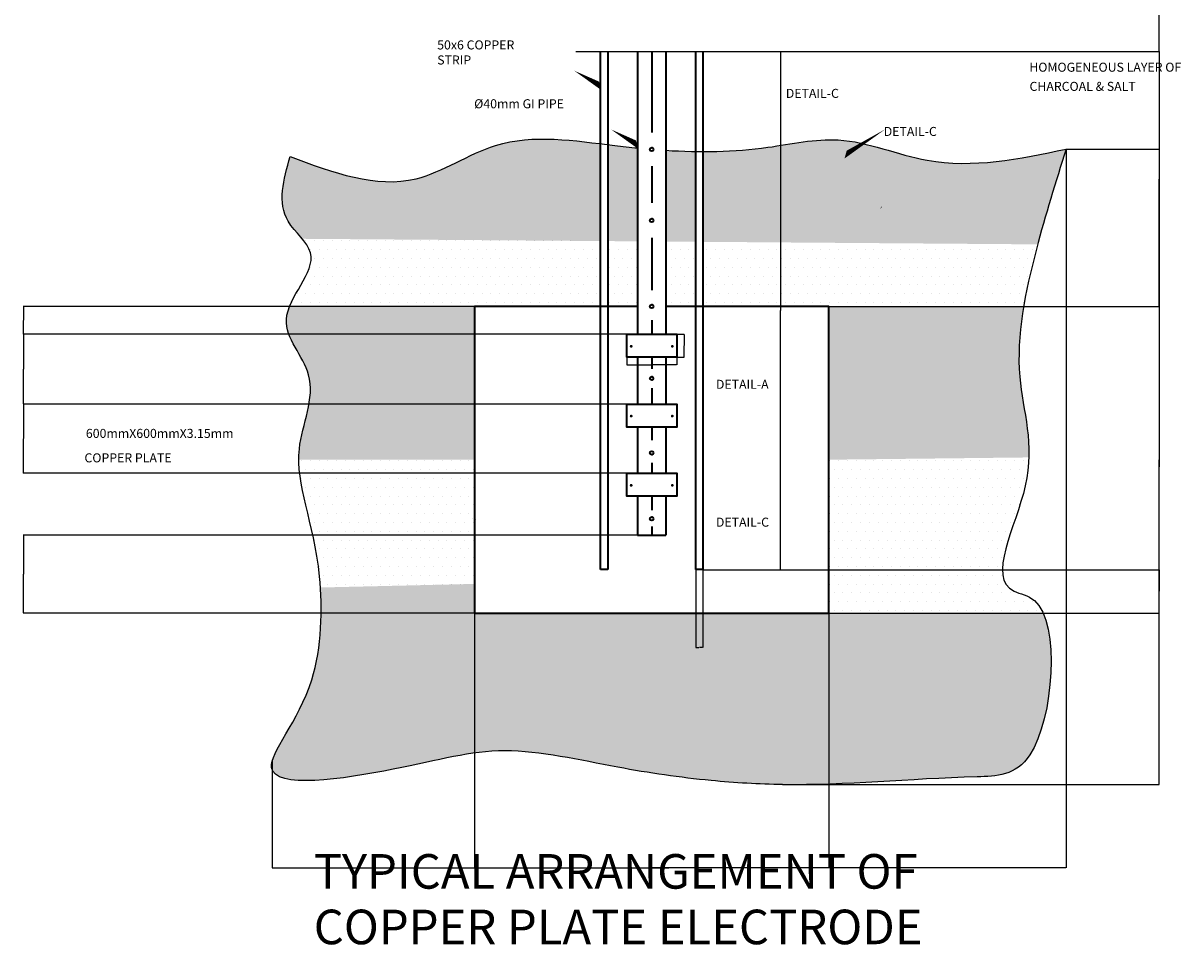
# Model space of a CAD drawing. Units: inches. Extents: x -514 to 1130, y -1450 to 978.
# Tile 1 of 2: x -514 to 1130, y -1450 to -141. Entities that reach past the tile are written whole.
import ezdxf

# ---------------------------------------------------------------- set-up
doc = ezdxf.new("R2010")
doc.units = ezdxf.units.IN
doc.header["$MEASUREMENT"] = 0
for name, color, linetype, lineweight in [('A-ANNO-DIMS', 2, 'Continuous', 18), ('C-TOPO', 3, 'Continuous', 25), ('C-TOPO-PATT', 252, 'Continuous', 13), ('E-ANNO-LEAD', 2, 'Continuous', 18), ('E-ANNO-TEXT', 7, 'Continuous', 18), ('E-GRND', 1, 'Continuous', 35)]:
    doc.layers.add(name, color=color, linetype=linetype, lineweight=lineweight)
doc.styles.get("Standard").update_dxf_attribs({"font": 'arial.ttf'})
doc.dimstyles.get("Standard").update_dxf_attribs({"dimtxt": 0.18, "dimasz": 0.18, "dimexe": 0.18, "dimexo": 0.0625, "dimgap": 0.09, "dimtad": 0, "dimtih": 1, "dimtoh": 1, "dimdec": 4, "dimzin": 0, "dimdsep": 46, "dimtxsty": 'Standard', "dimcen": 0.09, "dimadec": 0, "dimazin": 0, "dimtfac": 1, "dimtdec": 4, "dimtofl": 0, "dimtmove": 0, "dimatfit": 3, "dimfxl": 1, "dimtolj": 1, "dimtzin": 0, "dimarcsym": 0})

# ---------------------------------------------------------------- blocks, each defined once
blk = doc.blocks.new('CLAMP-PIPE')
blk.add_lwpolyline([(342.9, -582.6), (413.9, -582.6), (413.9, -615.2), (342.9, -615.2)], close=True)
at = {"const_width": 1.95}
for points in [[(348.3, -599.7, 1), (350.3, -599.7, 1)], [(406.7, -599.7, 1), (408.6, -599.7, 1)]]:
    blk.add_lwpolyline(points, format="xyb", close=True, dxfattribs=at)
blk = doc.blocks.new('COPPER-STRIP-50X6')
blk.add_line((10, 0), (0, 0))
for points in [[(0, 0), (0, 736)], [(10, 736), (10, 0)]]:
    blk.add_lwpolyline(points)
blk = doc.blocks.new('*D3')
at = {"layer": 'A-ANNO-DIMS', "color": 0, "lineweight": -2, "transparency": 16777216}
for p, q in [((342.9, -615.3), (342.9, -626)), ((413.9, -615.3), (413.9, -626)), ((343.1, -625.8), (377.1, -625.8)), ((413.7, -625.8), (379.7, -625.8))]:
    blk.add_line(p, q, dxfattribs=at)
at = {"layer": 'A-ANNO-DIMS', "color": 0, "transparency": 16777216}
for points in [[(343.1, -625.8), (343.1, -625.9), (342.9, -625.8)], [(413.7, -625.8), (413.7, -625.9), (413.9, -625.8)]]:
    blk.add_solid(points, dxfattribs=at)
at = {"layer": 'Defpoints', "color": 0, "transparency": 16777216}
for p in [(342.9, -615.2), (413.9, -615.2), (413.9, -625.8)]:
    blk.add_point(p, dxfattribs=at)
at = {"layer": 'A-ANNO-DIMS', "color": 0, "transparency": 16777216, "insert": (378.4, -625.8), "char_height": 0.18, "attachment_point": 5}
blk.add_mtext('\\A1;PIPE CLAMP 71 TYP.', dxfattribs=at)
blk = doc.blocks.new('*D4')
at = {"layer": 'A-ANNO-DIMS', "color": 0, "lineweight": -2, "transparency": 16777216}
for p, q in [((413.9, -582.6), (424.7, -582.6)), ((424.5, -582.8), (424.5, -598.7)), ((424.5, -615), (424.5, -599.1)), ((413.9, -615.2), (424.7, -615.2))]:
    blk.add_line(p, q, dxfattribs=at)
at = {"layer": 'A-ANNO-DIMS', "color": 0, "transparency": 16777216}
for points in [[(424.5, -582.8), (424.5, -582.8), (424.5, -582.6)], [(424.5, -615), (424.5, -615), (424.5, -615.2)]]:
    blk.add_solid(points, dxfattribs=at)
at = {"layer": 'Defpoints', "color": 0, "transparency": 16777216}
for p in [(413.9, -582.6), (424.5, -582.6), (413.9, -615.2)]:
    blk.add_point(p, dxfattribs=at)
at = {"layer": 'A-ANNO-DIMS', "color": 0, "transparency": 16777216, "insert": (424.5, -598.9), "char_height": 0.18, "attachment_point": 5}
blk.add_mtext('\\A1;33 TYP.', dxfattribs=at)
blk = doc.blocks.new('*D5')
at = {"layer": 'A-ANNO-DIMS', "color": 0, "lineweight": -2, "transparency": 16777216}
for p, q in [((451, -180.9), (561.5, -180.9)), ((561.3, -181.1), (561.3, -548.7)), ((561.3, -916.7), (561.3, -549.1)), ((451, -916.9), (561.5, -916.9))]:
    blk.add_line(p, q, dxfattribs=at)
at = {"layer": 'A-ANNO-DIMS', "color": 0, "transparency": 16777216}
for points in [[(561.3, -181.1), (561.3, -181.1), (561.3, -180.9)], [(561.3, -916.7), (561.3, -916.7), (561.3, -916.9)]]:
    blk.add_solid(points, dxfattribs=at)
at = {"layer": 'Defpoints', "color": 0, "transparency": 16777216}
for p in [(450.9, -180.9), (561.3, -180.9), (450.9, -916.9)]:
    blk.add_point(p, dxfattribs=at)
at = {"layer": 'A-ANNO-DIMS', "color": 0, "transparency": 16777216, "insert": (561.3, -548.9), "char_height": 0.18, "attachment_point": 5}
blk.add_mtext('\\A1;50X6 COPPER STRIP 736 TYP.', dxfattribs=at)
blk = doc.blocks.new('*D6')
at = {"layer": 'A-ANNO-DIMS', "color": 0, "lineweight": -2, "transparency": 16777216}
for p, q in [((440.9, -917), (440.9, -1027.5)), ((450.9, -917), (450.9, -1027.5)), ((441.1, -1027.3), (445.4, -1027.3)), ((450.7, -1027.3), (446.4, -1027.3))]:
    blk.add_line(p, q, dxfattribs=at)
at = {"layer": 'A-ANNO-DIMS', "color": 0, "transparency": 16777216}
for points in [[(441.1, -1027.3), (441.1, -1027.3), (440.9, -1027.3)], [(450.7, -1027.3), (450.7, -1027.3), (450.9, -1027.3)]]:
    blk.add_solid(points, dxfattribs=at)
at = {"layer": 'Defpoints', "color": 0, "transparency": 16777216}
for p in [(440.9, -916.9), (450.9, -916.9), (450.9, -1027.3)]:
    blk.add_point(p, dxfattribs=at)
at = {"layer": 'A-ANNO-DIMS', "color": 0, "transparency": 16777216, "insert": (445.9, -1027.3), "char_height": 0.18, "attachment_point": 5}
blk.add_mtext('\\A1;10 TYP.', dxfattribs=at)
blk = doc.blocks.new('*D22')
at = {"layer": 'A-ANNO-DIMS', "color": 0, "lineweight": -2, "transparency": 16777216}
for p, q in [((491.3, 109.1), (1099, 109.1)), ((1098.9, 108.9), (1098.9, -35.7)), ((1098.9, -180.7), (1098.9, -36.1)), ((491.3, -180.9), (1099, -180.9))]:
    blk.add_line(p, q, dxfattribs=at)
at = {"layer": 'A-ANNO-DIMS', "color": 0, "transparency": 16777216}
for points in [[(1098.8, 108.9), (1098.9, 108.9), (1098.9, 109.1)], [(1098.8, -180.7), (1098.9, -180.7), (1098.9, -180.9)]]:
    blk.add_solid(points, dxfattribs=at)
at = {"layer": 'Defpoints', "color": 0, "transparency": 16777216}
for p in [(491.2, 109.1), (491.2, -180.9), (1098.9, -180.9)]:
    blk.add_point(p, dxfattribs=at)
at = {"layer": 'A-ANNO-DIMS', "color": 0, "transparency": 16777216, "insert": (1098.9, -35.9), "char_height": 0.18, "attachment_point": 5}
blk.add_mtext('\\A1;290', dxfattribs=at)
blk = doc.blocks.new('*D26')
at = {"layer": 'A-ANNO-DIMS', "color": 0, "lineweight": -2, "transparency": 16777216}
for p, q in [((126.9, -978.5), (126.9, -1340.3)), ((629.9, -978.5), (629.9, -1340.3)), ((127.1, -1340.1), (378.1, -1340.1)), ((629.7, -1340.1), (378.7, -1340.1))]:
    blk.add_line(p, q, dxfattribs=at)
at = {"layer": 'A-ANNO-DIMS', "color": 0, "transparency": 16777216}
for points in [[(127.1, -1340), (127.1, -1340.1), (126.9, -1340.1)], [(629.7, -1340), (629.7, -1340.1), (629.9, -1340.1)]]:
    blk.add_solid(points, dxfattribs=at)
at = {"layer": 'Defpoints', "color": 0, "transparency": 16777216}
for p in [(126.9, -978.5), (629.9, -978.5), (629.9, -1340.1)]:
    blk.add_point(p, dxfattribs=at)
at = {"layer": 'A-ANNO-DIMS', "color": 0, "transparency": 16777216, "insert": (378.4, -1340.1), "char_height": 0.18, "attachment_point": 5}
blk.add_mtext('\\A1;503', dxfattribs=at)
blk = doc.blocks.new('*D27')
at = {"layer": 'A-ANNO-DIMS', "color": 0, "lineweight": -2, "transparency": 16777216}
for p, q in [((630, -543), (1099, -543)), ((1098.9, -543.2), (1098.9, -760.6)), ((1098.9, -978.3), (1098.9, -760.9)), ((630, -978.5), (1099, -978.5))]:
    blk.add_line(p, q, dxfattribs=at)
at = {"layer": 'A-ANNO-DIMS', "color": 0, "transparency": 16777216}
for points in [[(1098.8, -543.2), (1098.9, -543.2), (1098.9, -543)], [(1098.8, -978.3), (1098.9, -978.3), (1098.9, -978.5)]]:
    blk.add_solid(points, dxfattribs=at)
at = {"layer": 'Defpoints', "color": 0, "transparency": 16777216}
for p in [(629.9, -543), (629.9, -978.5), (1098.9, -978.5)]:
    blk.add_point(p, dxfattribs=at)
at = {"layer": 'A-ANNO-DIMS', "color": 0, "transparency": 16777216, "insert": (1098.9, -760.8), "char_height": 0.18, "attachment_point": 5}
blk.add_mtext('\\A1;435.4', dxfattribs=at)
blk = doc.blocks.new('*D28')
at = {"layer": 'A-ANNO-DIMS', "color": 0, "lineweight": -2, "transparency": 16777216}
for p, q in [((491.3, -180.9), (1099, -180.9)), ((1098.9, -181.1), (1098.9, -361.8)), ((1098.9, -542.9), (1098.9, -362.2)), ((630, -543), (1099, -543))]:
    blk.add_line(p, q, dxfattribs=at)
at = {"layer": 'A-ANNO-DIMS', "color": 0, "transparency": 16777216}
for points in [[(1098.8, -181.1), (1098.9, -181.1), (1098.9, -180.9)], [(1098.8, -542.9), (1098.9, -542.9), (1098.9, -543)]]:
    blk.add_solid(points, dxfattribs=at)
at = {"layer": 'Defpoints', "color": 0, "transparency": 16777216}
for p in [(491.2, -180.9), (629.9, -543), (1098.9, -543)]:
    blk.add_point(p, dxfattribs=at)
at = {"layer": 'A-ANNO-DIMS', "color": 0, "transparency": 16777216, "insert": (1098.9, -362), "char_height": 0.18, "attachment_point": 5}
blk.add_mtext('\\A1;362.14', dxfattribs=at)
blk = doc.blocks.new('*D29')
at = {"layer": 'A-ANNO-DIMS', "color": 0, "lineweight": -2, "transparency": 16777216}
for p, q in [((451, -916.9), (1099, -916.9)), ((1098.9, -917.1), (1098.9, -947.5)), ((1098.9, -978.3), (1098.9, -947.9)), ((630, -978.5), (1099, -978.5))]:
    blk.add_line(p, q, dxfattribs=at)
at = {"layer": 'A-ANNO-DIMS', "color": 0, "transparency": 16777216}
for points in [[(1098.8, -917.1), (1098.9, -917.1), (1098.9, -916.9)], [(1098.8, -978.3), (1098.9, -978.3), (1098.9, -978.5)]]:
    blk.add_solid(points, dxfattribs=at)
at = {"layer": 'Defpoints', "color": 0, "transparency": 16777216}
for p in [(450.9, -916.9), (629.9, -978.5), (1098.9, -978.5)]:
    blk.add_point(p, dxfattribs=at)
at = {"layer": 'A-ANNO-DIMS', "color": 0, "transparency": 16777216, "insert": (1098.9, -947.7), "char_height": 0.18, "attachment_point": 5}
blk.add_mtext('\\A1;61.58', dxfattribs=at)
blk = doc.blocks.new('*D30')
at = {"layer": 'A-ANNO-DIMS', "color": 0, "lineweight": -2, "transparency": 16777216}
for p, q in [((126.9, -543), (-513.8, -543)), ((-513.7, -543.2), (-513.7, -562.7)), ((-513.7, -582.5), (-513.7, -563)), ((342.9, -582.6), (-513.8, -582.6))]:
    blk.add_line(p, q, dxfattribs=at)
at = {"layer": 'A-ANNO-DIMS', "color": 0, "transparency": 16777216}
for points in [[(-513.7, -543.2), (-513.6, -543.2), (-513.7, -543)], [(-513.7, -582.5), (-513.6, -582.5), (-513.7, -582.6)]]:
    blk.add_solid(points, dxfattribs=at)
at = {"layer": 'Defpoints', "color": 0, "transparency": 16777216}
for p in [(126.9, -543), (-513.7, -582.6), (342.9, -582.6)]:
    blk.add_point(p, dxfattribs=at)
at = {"layer": 'A-ANNO-DIMS', "color": 0, "transparency": 16777216, "insert": (-513.7, -562.8), "char_height": 0.18, "attachment_point": 5}
blk.add_mtext('\\A1;39.594', dxfattribs=at)
blk = doc.blocks.new('*D31')
at = {"layer": 'A-ANNO-DIMS', "color": 0, "lineweight": -2, "transparency": 16777216}
for p, q in [((342.9, -582.6), (-513.8, -582.6)), ((-513.7, -582.8), (-513.7, -632)), ((-513.7, -681.6), (-513.7, -632.4)), ((342.9, -681.8), (-513.8, -681.8))]:
    blk.add_line(p, q, dxfattribs=at)
at = {"layer": 'A-ANNO-DIMS', "color": 0, "transparency": 16777216}
for points in [[(-513.7, -582.8), (-513.6, -582.8), (-513.7, -582.6)], [(-513.7, -681.6), (-513.6, -681.6), (-513.7, -681.8)]]:
    blk.add_solid(points, dxfattribs=at)
at = {"layer": 'Defpoints', "color": 0, "transparency": 16777216}
for p in [(342.9, -582.6), (-513.7, -681.8), (342.9, -681.8)]:
    blk.add_point(p, dxfattribs=at)
at = {"layer": 'A-ANNO-DIMS', "color": 0, "transparency": 16777216, "insert": (-513.7, -632.2), "char_height": 0.18, "attachment_point": 5}
blk.add_mtext('\\A1;99.12', dxfattribs=at)
blk = doc.blocks.new('*D32')
at = {"layer": 'A-ANNO-DIMS', "color": 0, "lineweight": -2, "transparency": 16777216}
for p, q in [((342.9, -681.8), (-513.8, -681.8)), ((-513.7, -681.9), (-513.7, -730.8)), ((-513.7, -779.9), (-513.7, -731.1)), ((342.9, -780.1), (-513.8, -780.1))]:
    blk.add_line(p, q, dxfattribs=at)
at = {"layer": 'A-ANNO-DIMS', "color": 0, "transparency": 16777216}
for points in [[(-513.7, -681.9), (-513.6, -681.9), (-513.7, -681.8)], [(-513.7, -779.9), (-513.6, -779.9), (-513.7, -780.1)]]:
    blk.add_solid(points, dxfattribs=at)
at = {"layer": 'Defpoints', "color": 0, "transparency": 16777216}
for p in [(342.9, -681.8), (-513.7, -780.1), (342.9, -780.1)]:
    blk.add_point(p, dxfattribs=at)
at = {"layer": 'A-ANNO-DIMS', "color": 0, "transparency": 16777216, "insert": (-513.7, -730.9), "char_height": 0.18, "attachment_point": 5}
blk.add_mtext('\\A1;98.37', dxfattribs=at)
blk = doc.blocks.new('*D33')
at = {"layer": 'A-ANNO-DIMS', "color": 0, "lineweight": -2, "transparency": 16777216}
for p, q in [((358.3, -868.1), (-513.8, -868.1)), ((-513.7, -868.3), (-513.7, -923.1)), ((-513.7, -978.3), (-513.7, -923.5)), ((126.9, -978.5), (-513.8, -978.5))]:
    blk.add_line(p, q, dxfattribs=at)
at = {"layer": 'A-ANNO-DIMS', "color": 0, "transparency": 16777216}
for points in [[(-513.7, -868.3), (-513.6, -868.3), (-513.7, -868.1)], [(-513.7, -978.3), (-513.6, -978.3), (-513.7, -978.5)]]:
    blk.add_solid(points, dxfattribs=at)
at = {"layer": 'Defpoints', "color": 0, "transparency": 16777216}
for p in [(358.4, -868.1), (-513.7, -978.5), (126.9, -978.5)]:
    blk.add_point(p, dxfattribs=at)
at = {"layer": 'A-ANNO-DIMS', "color": 0, "transparency": 16777216, "insert": (-513.7, -923.3), "char_height": 0.18, "attachment_point": 5}
blk.add_mtext('\\A1;110.35', dxfattribs=at)
blk = doc.blocks.new('*D34')
at = {"layer": 'A-ANNO-DIMS', "color": 0, "lineweight": -2, "transparency": 16777216}
for p, q in [((966.7, -319.9), (966.7, -1340.3)), ((-160.5, -1188.9), (-160.5, -1340.3)), ((-160.4, -1340.1), (402.6, -1340.1)), ((966.5, -1340.1), (403.6, -1340.1))]:
    blk.add_line(p, q, dxfattribs=at)
at = {"layer": 'A-ANNO-DIMS', "color": 0, "transparency": 16777216}
for points in [[(-160.4, -1340), (-160.4, -1340.1), (-160.5, -1340.1)], [(966.5, -1340), (966.5, -1340.1), (966.7, -1340.1)]]:
    blk.add_solid(points, dxfattribs=at)
at = {"layer": 'Defpoints', "color": 0, "transparency": 16777216}
for p in [(966.7, -319.8), (-160.5, -1188.9), (966.7, -1340.1)]:
    blk.add_point(p, dxfattribs=at)
at = {"layer": 'A-ANNO-DIMS', "color": 0, "transparency": 16777216, "insert": (403.1, -1340.1), "char_height": 0.18, "attachment_point": 5}
blk.add_mtext('\\A1;1127.3', dxfattribs=at)
blk = doc.blocks.new('*D35')
at = {"layer": 'A-ANNO-DIMS', "color": 0, "lineweight": -2, "transparency": 16777216}
for p, q in [((966.8, -319.8), (1099, -319.8)), ((1098.9, -320), (1098.9, -770.8)), ((1098.9, -1221.9), (1098.9, -771.1)), ((564.3, -1222.1), (1099, -1222.1))]:
    blk.add_line(p, q, dxfattribs=at)
at = {"layer": 'A-ANNO-DIMS', "color": 0, "transparency": 16777216}
for points in [[(1098.8, -320), (1098.9, -320), (1098.9, -319.8)], [(1098.8, -1221.9), (1098.9, -1221.9), (1098.9, -1222.1)]]:
    blk.add_solid(points, dxfattribs=at)
at = {"layer": 'Defpoints', "color": 0, "transparency": 16777216}
for p in [(966.7, -319.8), (564.2, -1222.1), (1098.9, -1222.1)]:
    blk.add_point(p, dxfattribs=at)
at = {"layer": 'A-ANNO-DIMS', "color": 0, "transparency": 16777216, "insert": (1098.9, -770.9), "char_height": 0.18, "attachment_point": 5}
blk.add_mtext('\\A1;902.3', dxfattribs=at)

msp = doc.modelspace()

# ---------------------------------------------------------------- hatches: boundary and pattern name
at = {"layer": 'C-TOPO-PATT'}
h = msp.add_hatch(dxfattribs=at)
h.set_pattern_fill('HEX', color=256, scale=60)
edge = h.paths.add_edge_path()
edge.add_spline(control_points=[(305.9114, -312.0843), (255.1866, -305.7764), (162.1476, -294.9931), (28.4437, -390.9059), (-73.917, -352.9564), (-135.0278, -330.3001), (-144.1924, -363.0231), (-156.3777, -406.5315), (-124.607, -439.0103), (-117.9173, -447.0708)], knot_values=[2558.576308896, 2558.576308896, 2558.576308896, 2558.576308896, 2707.976967101, 2830.531301613, 3012.092961341, 3012.092961341, 3012.092961341, 3104.06054613, 3134.372709078, 3134.372709078, 3134.372709078, 3134.372709078], degree=3, periodic=0)
edge.add_line((-117.9173, -447.0708), (305.9114, -450.2757))
edge.add_line((305.9114, -450.2757), (305.9114, -312.0843))
edge = h.paths.add_edge_path()
edge.add_spline(control_points=[(926.4196, -454.9679), (938.7739, -408.7375), (952.75, -364.2656), (966.726, -319.7938)], knot_values=[0, 0, 0, 0, 141.175598989, 141.175598989, 141.175598989, 141.175598989], degree=3, periodic=0)
edge.add_spline(control_points=[(966.726, -319.7938), (900.3974, -333.5642), (790.659, -356.3469), (653.584, -294.712), (545.7543, -319.617), (481.7435, -323.2948), (450.9114, -323.2008)], knot_values=[3278.625747001, 3278.625747001, 3278.625747001, 3278.625747001, 3476.465744458, 3605.945645556, 3706.416880749, 3799.313199321, 3799.313199321, 3799.313199321, 3799.313199321], degree=3, periodic=0)
edge.add_line((450.9114, -323.2008), (450.9114, -451.3722))
edge.add_line((450.9114, -451.3722), (926.4196, -454.9679))
edge = h.paths.add_edge_path()
edge.add_spline(control_points=[(358.4114, -318.1134), (347.593, -317.0483), (333.4463, -315.4827), (319.2248, -313.738), (315.9114, -313.3278)], knot_values=[3144.196564241, 3144.196564241, 3144.196564241, 3144.196564241, 3176.40431904, 3186.1768941, 3186.1768941, 3186.1768941, 3186.1768941], degree=3, periodic=0)
edge.add_line((315.9114, -313.3278), (315.9114, -450.3514))
edge.add_line((315.9114, -450.3514), (358.4114, -450.6727))
edge.add_line((358.4114, -450.6727), (358.4114, -318.1134))
edge = h.paths.add_edge_path()
edge.add_spline(control_points=[(440.9114, -323.106), (426.7733, -322.8825), (412.6134, -322.2848), (398.4114, -321.3836)], knot_values=[3226.015463929, 3226.015463929, 3226.015463929, 3226.015463929, 3268.585625788, 3268.585625788, 3268.585625788, 3268.585625788], degree=3, periodic=0)
edge.add_line((398.4114, -321.3836), (398.4114, -450.9752))
edge.add_line((398.4114, -450.9752), (440.9114, -451.2966))
edge.add_line((440.9114, -451.2966), (440.9114, -323.106))
edge = h.paths.add_edge_path()
edge.add_spline(control_points=[(913.9671, -757.5216), (915.1505, -715.9834), (894.9887, -650.219), (900.9088, -576.9646), (906.5871, -543.0396)], knot_values=[229.379387274, 229.379387274, 229.379387274, 229.379387274, 348.036394784, 449.372068737, 449.372068737, 449.372068737, 449.372068737], degree=3, periodic=0)
edge.add_line((906.5871, -543.0396), (629.9001, -543.0396))
edge.add_line((629.9001, -543.0396), (629.9001, -760.755))
edge.add_line((629.9001, -760.755), (913.9671, -757.5216))
edge = h.paths.add_edge_path()
edge.add_line((126.9226, -543.0396), (-135.6988, -543.0396))
edge.add_spline(control_points=[(-135.6988, -543.0396), (-138.2127, -549.2256), (-147.596, -582.6879), (-84.3642, -644.6462), (-120.7631, -715.3201), (-122.6941, -755.6416), (-122.6721, -760.8136)], knot_values=[2227.362231503, 2227.362231503, 2227.362231503, 2227.362231503, 2246.486456495, 2331.366553539, 2437.248834262, 2452.791404045, 2452.791404045, 2452.791404045, 2452.791404045], degree=3, periodic=0)
edge.add_line((-122.6721, -760.8136), (126.9226, -760.755))
edge.add_line((126.9226, -760.755), (126.9226, -543.0396))
h = msp.add_hatch(dxfattribs=at)
h.set_pattern_fill('DOTS', color=256, scale=200)
edge = h.paths.add_edge_path()
edge.add_line((305.9114, -450.2757), (-117.9173, -447.0708))
edge.add_spline(control_points=[(-117.9173, -447.0708), (-112.5404, -453.5495), (-92.5209, -481.7059), (-124.9959, -516.7024), (-135.6988, -543.0396)], knot_values=[2452.791404045, 2452.791404045, 2452.791404045, 2452.791404045, 2477.154815033, 2558.576308896, 2558.576308896, 2558.576308896, 2558.576308896], degree=3, periodic=0)
edge.add_line((-135.6988, -543.0396), (126.9226, -543.0396))
edge.add_line((126.9226, -543.0396), (305.9114, -543.0396))
edge.add_line((305.9114, -543.0396), (305.9114, -450.2757))
h = msp.add_hatch(dxfattribs=at)
h.set_pattern_fill('DOTS', color=256, scale=200)
edge = h.paths.add_edge_path()
edge.add_line((126.9226, -760.755), (-122.6721, -760.8136))
edge.add_spline(control_points=[(-122.6721, -760.8136), (-122.4736, -807.4113), (-98.8319, -858.3093), (-92.2406, -936.8365), (-91.8839, -942.218)], knot_values=[2077.226003647, 2077.226003647, 2077.226003647, 2077.226003647, 2217.258049419, 2227.362231503, 2227.362231503, 2227.362231503, 2227.362231503], degree=3, periodic=0)
edge.add_line((-91.8839, -942.218), (126.9226, -937.1171))
edge.add_line((126.9226, -937.1171), (126.9226, -760.755))
edge = h.paths.add_edge_path()
edge.add_spline(control_points=[(934.1175, -978.4705), (930.7904, -971.0144), (919.2875, -954.0087), (844.5148, -943.3117), (905.8885, -838.7284), (913.603, -770.3031), (913.9671, -757.5216)], knot_values=[449.372068737, 449.372068737, 449.372068737, 449.372068737, 466.426239302, 497.199581115, 647.743126183, 684.254466767, 684.254466767, 684.254466767, 684.254466767], degree=3, periodic=0)
edge.add_line((913.9671, -757.5216), (629.9001, -760.755))
edge.add_line((629.9001, -760.755), (629.9001, -978.4705))
edge.add_line((629.9001, -978.4705), (934.1175, -978.4705))
edge = h.paths.add_edge_path()
edge.add_spline(control_points=[(906.5871, -543.0396), (911.1503, -515.7764), (918.1572, -486.1206), (925.8274, -457.184), (926.4196, -454.9679)], knot_values=[141.175598989, 141.175598989, 141.175598989, 141.175598989, 222.611902009, 229.379387274, 229.379387274, 229.379387274, 229.379387274], degree=3, periodic=0)
edge.add_line((926.4196, -454.9679), (450.9114, -451.3722))
edge.add_line((450.9114, -451.3722), (450.9114, -543.0396))
edge.add_line((450.9114, -543.0396), (629.9001, -543.0396))
edge.add_line((629.9001, -543.0396), (906.5871, -543.0396))
h.paths.add_polyline_path([(440.9114, -451.2966), (398.4114, -450.9752), (398.4114, -543.0396), (440.9114, -543.0396)])
h.paths.add_polyline_path([(358.4114, -450.6727), (315.9114, -450.3514), (315.9114, -543.0396), (358.4114, -543.0396)])
h = msp.add_hatch(dxfattribs=at)
h.set_pattern_fill('HEX', color=256, scale=60)
edge = h.paths.add_edge_path()
edge.add_spline(control_points=[(-91.8839, -942.218), (-89.0821, -984.4826), (-95.4593, -1104.845), (-224.3178, -1239.0629), (31.1239, -1200.9077), (163.9896, -1161.2999), (322.5805, -1198.0653), (451.365, -1216.9213), (623.7933, -1227.0137), (765.4968, -1211.2096), (936.7185, -1209.5718), (955.9045, -1027.2952), (934.1175, -978.4705)], knot_values=[684.254466767, 684.254466767, 684.254466767, 684.254466767, 763.608423146, 882.298593781, 1055.253603965, 1215.7522685, 1377.799282437, 1511.646302567, 1613.237961486, 1889.664797207, 1965.551324857, 2077.226003647, 2077.226003647, 2077.226003647, 2077.226003647], degree=3, periodic=0)
edge.add_line((934.1175, -978.4705), (629.9001, -978.4705))
edge.add_line((629.9001, -978.4705), (126.9226, -978.4705))
edge.add_line((126.9226, -978.4705), (126.9226, -937.1171))
edge.add_line((126.9226, -937.1171), (-91.8839, -942.218))

# ---------------------------------------------------------------- linework, layer by layer
at = {"layer": 'C-TOPO'}
msp.add_line((270.9153, -180.8997), (491.2068, -180.8997), dxfattribs=at)
for points, knots in [([(966.726, -319.7938), (952.08, -366.3975), (919.34, -470.5764), (884.9403, -638.4925), (939.3204, -781.759), (844.5148, -943.3117), (961.3814, -960.0307), (943.0119, -1209.5116), (765.4968, -1211.2096), (623.7933, -1227.0137), (451.365, -1216.9213), (322.5805, -1198.0653), (163.9896, -1161.2999), (31.1239, -1200.9077), (-224.3178, -1239.0629), (-91.9498, -1101.1896), (-86.0856, -875.5702), (-145.4693, -763.2908), (-84.3642, -644.6462), (-172.1255, -558.6523), (-76.8768, -476.4137), (-158.8055, -415.2003), (-144.1924, -363.0231), (-135.0278, -330.3001), (-73.917, -352.9564), (28.4437, -390.9059), (167.9249, -290.8487), (279.7902, -309.5449), (347.593, -317.0483), (358.4114, -318.1134)], [0, 0, 0, 0, 147.943084254, 330.715061227, 485.88340932, 636.426954389, 667.200296202, 795.929145557, 871.815673207, 1148.242508928, 1249.834167847, 1383.681187977, 1545.728201914, 1706.226866449, 1879.181876633, 1997.872047268, 2087.330185731, 2242.904801285, 2348.787082008, 2433.667179053, 2534.212897908, 2588.888471844, 2680.856056633, 2680.856056633, 2680.856056633, 2862.417716362, 2984.972050874, 3153.969139301, 3186.1768941, 3186.1768941, 3186.1768941, 3186.1768941]), ([(398.4114, -321.3836), (446.9546, -324.4642), (528.1827, -323.6755), (653.584, -294.712), (790.659, -356.3469), (900.3974, -333.5642), (966.726, -319.7938)], [3226.015463929, 3226.015463929, 3226.015463929, 3226.015463929, 3371.522065573, 3471.993300766, 3601.473201864, 3799.313199321, 3799.313199321, 3799.313199321, 3799.313199321])]:
    msp.add_open_spline(points, degree=3, knots=knots, dxfattribs=at)
at = {"layer": 'E-ANNO-LEAD'}
for points in [[(306.9307, -236.0174, 0, 13.2101, 0), (296.1174, -220.5728, 0, 0, 0), (211.8959, -183.3957, 0, 0, 0), (114.3664, -183.3957, 0, 0, 0)], [(513.0969, -202.0689, 0, 13.2101, 0), (523.9103, -217.5136, 0, 0, 0), (550.1315, -254.0774, 0, 0, 0), (647.661, -254.0774, 0, 0, 0)], [(652.1655, -333.0903, 0, 13.2101, 0), (662.9788, -317.6456, 0, 0, 0), (847.4535, -215.0215, 0, 0, 0), (944.983, -215.0215, 0, 0, 0)], [(704.8877, -402.7424, 0, 13.2101, 0), (715.701, -387.2977, 0, 0, 0), (847.4535, -215.0215, 0, 0, 0)], [(359.4307, -319.5693, 0, 13.2101, 0), (348.6174, -304.1247, 0, 0, 0), (264.3959, -266.9476, 0, 0, 0), (166.8664, -266.9476, 0, 0, 0)], [(413.8768, -615.1959, 0, 13.2101, 0), (424.6901, -630.6406, 0, 0, 0), (450.9114, -667.2044, 0, 0, 0), (548.4409, -667.2044, 0, 0, 0)], [(126.9226, -843.8562, 0, 13.2101, 0), (102.9288, -836.5065, 0, 0, 0), (-172.7726, -743.141, 0, 0, 0), (-395.658, -743.141, 0, 0, 0)], [(413.8768, -810.971, 0, 13.2101, 0), (424.6901, -826.4157, 0, 0, 0), (450.9114, -862.9795, 0, 0, 0), (548.4409, -862.9795, 0, 0, 0)]]:
    msp.add_lwpolyline(points, format="xyseb", dxfattribs=at)
at = {"layer": 'E-GRND'}
for p, q in [((358.4114, -180.8997), (358.4114, -582.6338)), ((378.4114, -180.8997), (378.4114, -295.9977)), ((398.4114, -180.8997), (398.4114, -582.6338)), ((378.4114, -343.9676), (378.4114, -396.1647)), ((378.4114, -445.4671), (378.4114, -520.1044)), ((378.4114, -562.7443), (378.4114, -582.6338)), ((358.4114, -615.1959), (358.4114, -681.7506)), ((378.4114, -615.1959), (378.4114, -631.6973)), ((398.4114, -615.1959), (398.4114, -681.7506)), ((378.4114, -659.1231), (378.4114, -681.7506)), ((358.4114, -714.3128), (358.4114, -780.1222)), ((378.4114, -714.3128), (378.4114, -733.1206)), ((398.4114, -714.3128), (398.4114, -780.1222)), ((378.4114, -765.1626), (378.4114, -780.1222)), ((358.4114, -812.6844), (358.4114, -868.1248)), ((378.4114, -812.6844), (378.4114, -832.6101)), ((398.4114, -812.6844), (398.4114, -868.1248)), ((358.4114, -868.1248), (398.4114, -868.1248)), ((378.4114, -855.5076), (378.4114, -868.1248))]:
    msp.add_line(p, q, dxfattribs=at)
msp.add_lwpolyline([(358.4114, -543.0396), (126.9226, -543.0396), (126.9226, -978.4705), (629.9001, -978.4705), (629.9001, -543.0396), (398.4114, -543.0396)], dxfattribs=at)
for centre in [(378.4114, -320.1316), (378.4114, -421.0047), (378.4114, -543.0515), (378.4114, -645.1767), (378.4114, -751.0529), (378.4114, -844.604)]:
    msp.add_circle(centre, 2.5732, dxfattribs=at)

# ---------------------------------------------------------------- block references
for name, p in [('COPPER-STRIP-50X6', (305.911, -916.888)), ('COPPER-STRIP-50X6', (440.911, -916.888)), ('CLAMP-PIPE', (0, 0)), ('CLAMP-PIPE', (0, -99.1168)), ('CLAMP-PIPE', (0, -197.4884))]:
    msp.add_blockref(name, p, dxfattribs=at)

# ---------------------------------------------------------------- texts
at = {"layer": 'E-ANNO-TEXT'}
for s, height, p in [('HOMOGENEOUS LAYER OF ', 12.829888, (914.5578, -209.8258)), ('CHARCOAL & SALT', 12.829888, (914.8657, -237.0407)), ('DETAIL-C', 12.82989, (568.8134, -246.9546)), ('DETAIL-C', 12.82989, (707.882, -301.0345)), ('DETAIL-A', 12.82989, (469.5933, -660.0816)), ('600mmX600mmX3.15mm', 12.829888, (-424.9454, -729.8067)), ('COPPER PLATE', 12.829888, (-427.0053, -764.5159)), ('DETAIL-C', 12.82989, (469.5933, -855.8566)), ('TYPICAL ARRANGEMENT OF', 49.111465, (-101.4554, -1369.8934)), ('COPPER PLATE ELECTRODE', 49.111465, (-101.4554, -1448.7866))]:
    msp.add_text(s, height=height, dxfattribs=at).set_placement(p)
at = {"layer": 'E-ANNO-TEXT', "char_height": 12.829888, "width": 218.032909, "attachment_point": 1}
for s, insert in [('50x6 COPPER\\PSTRIP', (73.8377, -165.3445)), ('%%C40mm GI PIPE', (126.3377, -248.8963))]:
    msp.add_mtext(s, dxfattribs=dict(at, insert=insert))

# ---------------------------------------------------------------- dimensions: what is measured, and where the dimension line sits
at = {"layer": 'A-ANNO-DIMS'}
for base, p1, p2, override, picture, middle in [((1098.8592, -180.8997), (491.2068, 109.1003), (491.2068, -180.8997), {"dimdec": 0, "dimlfac": 1, "dimrnd": 0, "dimzin": 0, "dimdsep": 46, "dimlunit": 2}, '*D22', (1098.8592, -35.8997)), ((1098.8592, -543.0396), (491.2068, -180.8997), (629.9001, -543.0396), {"dimdec": 2, "dimlfac": 1, "dimrnd": 0, "dimzin": 0, "dimdsep": 46, "dimlunit": 2}, '*D28', (1098.8592, -361.9696)), ((1098.8592, -1222.0775), (966.726, -319.7938), (564.2242, -1222.0775), {"dimdec": 1, "dimlfac": 1, "dimrnd": 0, "dimzin": 0, "dimdsep": 46, "dimlunit": 2}, '*D35', (1098.8592, -770.9357)), ((-513.658, -582.6338), (126.9226, -543.0396), (342.946, -582.6338), {"dimdec": 3, "dimlfac": 1, "dimrnd": 0, "dimzin": 0, "dimdsep": 46, "dimlunit": 2}, '*D30', (-513.658, -562.8367)), ((1098.8592, -978.4705), (629.9001, -543.0396), (629.9001, -978.4705), {"dimdec": 1, "dimlfac": 1, "dimrnd": 0, "dimzin": 0, "dimdsep": 46, "dimlunit": 2}, '*D27', (1098.8592, -760.755)), ((-513.658, -681.7506), (342.946, -582.6338), (342.946, -681.7506), {"dimdec": 2, "dimlfac": 1, "dimrnd": 0, "dimzin": 0, "dimdsep": 46, "dimlunit": 2}, '*D31', (-513.658, -632.1922)), ((-513.658, -780.1222), (342.946, -681.7506), (342.946, -780.1222), {"dimdec": 2, "dimlfac": 1, "dimrnd": 0, "dimzin": 0, "dimdsep": 46, "dimlunit": 2}, '*D32', (-513.658, -730.9364)), ((-513.658, -978.4705), (358.4114, -868.1248), (126.9226, -978.4705), {"dimdec": 2, "dimlfac": 1, "dimrnd": 0, "dimzin": 0, "dimdsep": 46, "dimlunit": 2}, '*D33', (-513.658, -923.2977)), ((1098.8592, -978.4705), (450.9114, -916.8879), (629.9001, -978.4705), {"dimdec": 2, "dimlfac": 1, "dimrnd": 0, "dimzin": 0, "dimdsep": 46, "dimlunit": 2}, '*D29', (1098.8592, -947.6792))]:
    dim = msp.add_linear_dim(base=base, p1=p1, p2=p2, angle=90, dimstyle='Standard', override=override, dxfattribs=at)
    dim.commit()
    dim.dimension.update_dxf_attribs({"geometry": picture, "text_midpoint": middle})
for base, p1, p2, text, picture, middle in [((561.3096, -180.8997), (450.9114, -916.8879), (450.9114, -180.8997), '50X6 COPPER STRIP <> TYP.', '*D5', (561.3096, -548.8938)), ((424.5164, -582.6338), (413.8768, -615.1959), (413.8768, -582.6338), '<> TYP.', '*D4', (424.5164, -598.9149))]:
    dim = msp.add_linear_dim(base=base, p1=p1, p2=p2, angle=90, text=text, dimstyle='Standard', override={"dimdec": 0, "dimrnd": 0, "dimzin": 0, "dimlunit": 2}, dxfattribs=at)
    dim.commit()
    dim.dimension.update_dxf_attribs({"geometry": picture, "text_midpoint": middle})
for base, p1, p2, override, picture, middle in [((966.726, -1340.0775), (-160.5338, -1188.8575), (966.726, -319.7938), {"dimdec": 1, "dimlfac": 1, "dimrnd": 0, "dimzin": 0, "dimdsep": 46, "dimlunit": 2}, '*D34', (403.0961, -1340.0775)), ((629.9001, -1340.0775), (126.9226, -978.4705), (629.9001, -978.4705), {"dimdec": 0, "dimlfac": 1, "dimrnd": 0, "dimzin": 0, "dimdsep": 46, "dimlunit": 2}, '*D26', (378.4114, -1340.0775))]:
    dim = msp.add_linear_dim(base=base, p1=p1, p2=p2, dimstyle='Standard', override=override, dxfattribs=at)
    dim.commit()
    dim.dimension.update_dxf_attribs({"geometry": picture, "text_midpoint": middle})
for base, p1, p2, text, picture, middle in [((413.8768, -625.8356), (342.946, -615.1959), (413.8768, -615.1959), 'PIPE CLAMP <> TYP.', '*D3', (378.4114, -625.8356)), ((450.9114, -1027.2862), (440.9114, -916.8879), (450.9114, -916.8879), '<> TYP.', '*D6', (445.9114, -1027.2862))]:
    dim = msp.add_linear_dim(base=base, p1=p1, p2=p2, text=text, dimstyle='Standard', override={"dimdec": 0, "dimrnd": 0, "dimzin": 0, "dimlunit": 2}, dxfattribs=at)
    dim.commit()
    dim.dimension.update_dxf_attribs({"geometry": picture, "text_midpoint": middle})

doc.saveas('drawing.dxf')
